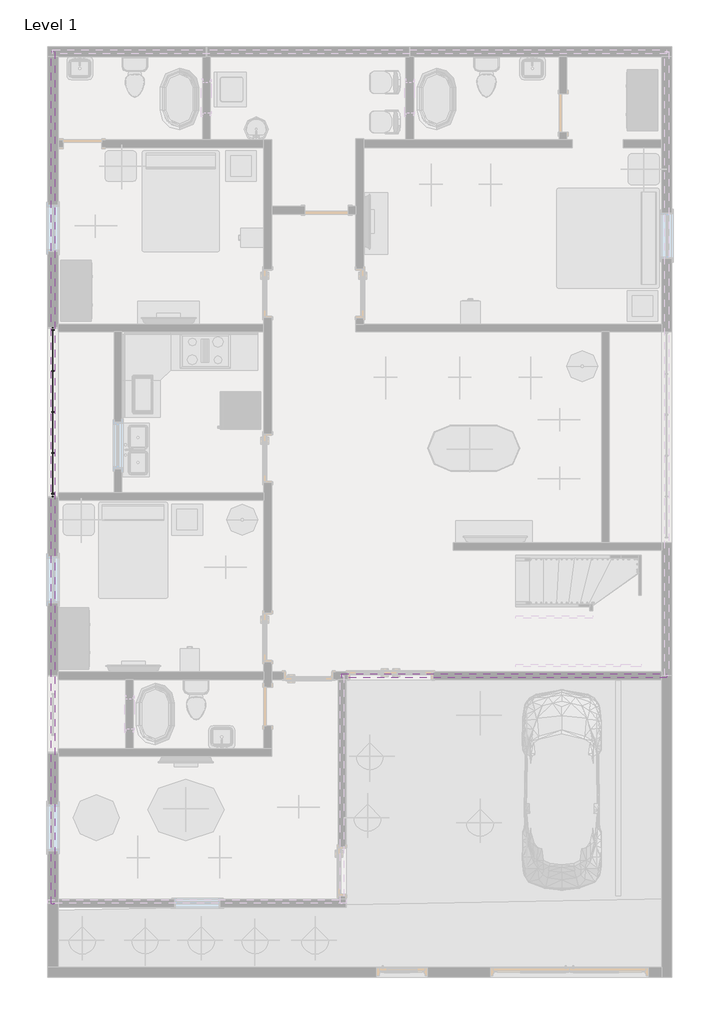
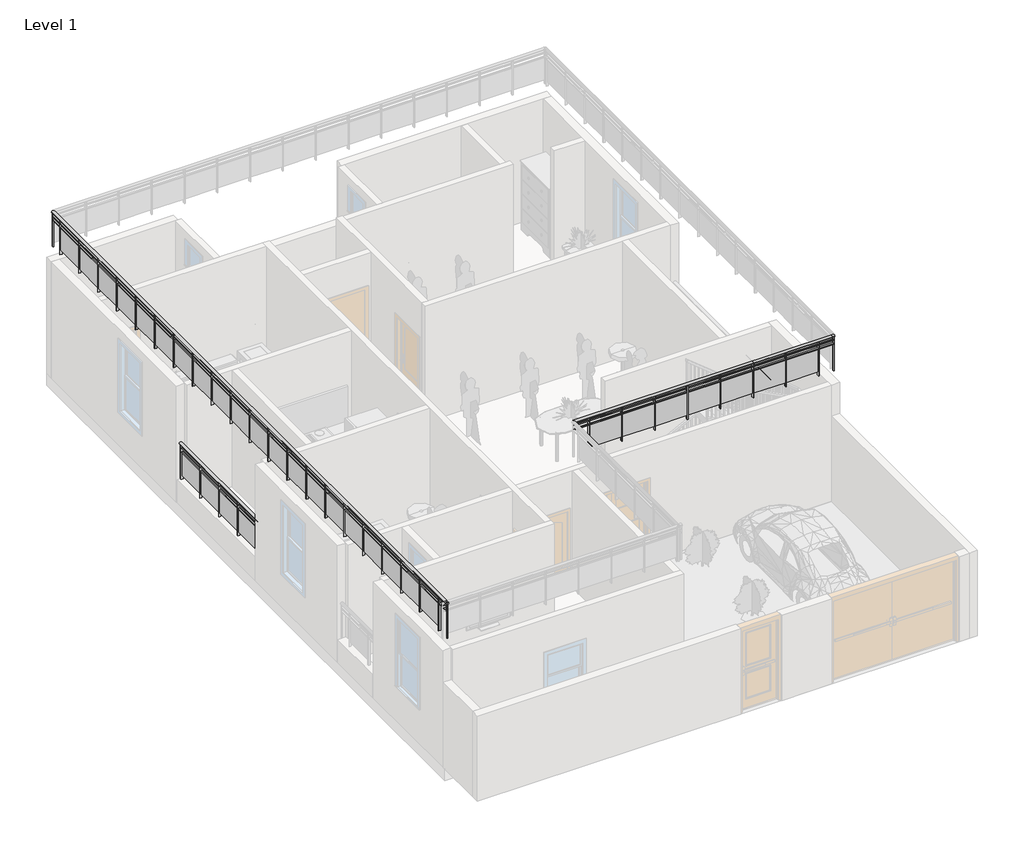
# One storey, part 3 of 6: 3 railings.
"""IFC4 building model written with IfcOpenShell, lengths in millimetres."""

from ifc_helpers import new_model, si_unit, point, frame, origin, place, context, project, spatial, polyline, ellipse_curve, trimmed, outline, extrude, element, save
from ifc_brep_helpers import plane_surface, extruded_surface, advanced_brep

model = new_model("IFC4")

# Units and contexts
model_context = context("Model", 3, world=origin())
ifc_project = project(units=[si_unit("LENGTHUNIT", "METRE", prefix="MILLI")], contexts=[model_context])

# Site, building, storey
site = spatial("IfcSite", under=ifc_project)
building = spatial("IfcBuilding", under=site)
storey = spatial("IfcBuildingStorey", under=building, Name="Level 1", Elevation=0.0)

# Railings
placement = place(None, origin())
element("IfcRailing", 1, ObjectType="Glass Panel - Bottom Fill", at=placement, inside=storey, context=model_context, shape_type="SolidModel", body=[
    advanced_brep(
    [(-14543.6841185, 4912.4271763, 1524.0), (-14467.4841185, 4912.4271763, 1524.0), (-14543.6841185, 8277.9271763, 1524.0), (-14467.4841185, 8277.9271763, 1524.0)],
    [
        (0, 1, ellipse_curve(frame((-14505.5841185, 4912.4271763, 1524.0), z_axis=(0.0, -1.0, 0.0), x_axis=(1.0, 0.0, 0.0)), 38.1, 28.575)),
        (1, 0, ellipse_curve(frame((-14505.5841185, 4912.4271763, 1524.0), z_axis=(0.0, -1.0, 0.0), x_axis=(1.0, 0.0, 0.0)), 38.1, 28.575)),
        (2, 3, ellipse_curve(frame((-14505.5841185, 8277.9271763, 1524.0), z_axis=(0.0, 1.0, 0.0), x_axis=(1.0, 0.0, 0.0)), 38.1, 28.575)),
        (3, 2, ellipse_curve(frame((-14505.5841185, 8277.9271763, 1524.0), z_axis=(0.0, 1.0, 0.0), x_axis=(1.0, 0.0, 0.0)), 38.1, 28.575)),
        (0, 2),
        (3, 1),
    ],
    [
        plane_surface(frame((-14505.5841185, 4912.4271763, 1524.0), z_axis=(0.0, -1.0, 0.0), x_axis=(0.0, 0.0, 1.0))),
        plane_surface(frame((-14505.5841185, 8277.9271763, 1524.0), z_axis=(0.0, 1.0, 0.0), x_axis=(0.0, 0.0, 1.0))),
        extruded_surface(trimmed(ellipse_curve(frame((-14505.5841185, 8277.9271763, 1524.0), z_axis=(0.0, -1.0, 0.0), x_axis=(1.0, 0.0, 0.0)), 38.1, 28.575), [point((-14543.6841185, 8277.9271763, 1524.0))], [point((-14467.4841185, 8277.9271763, 1524.0))], True, "CARTESIAN"), (0.0, -3365.5, 0.0), 3365.5),
        extruded_surface(trimmed(ellipse_curve(frame((-14505.5841185, 8277.9271763, 1524.0), z_axis=(0.0, -1.0, 0.0), x_axis=(1.0, 0.0, 0.0)), 38.1, 28.575), [point((-14467.4841185, 8277.9271763, 1524.0))], [point((-14543.6841185, 8277.9271763, 1524.0))], True, "CARTESIAN"), (0.0, -3365.5, 0.0), 3365.5),
    ],
    [
        (0, [[1, 2]]),
        (1, [[3, 4]]),
        (2, [[-1, 5, -4, 6]]),
        (3, [[-2, -6, -3, -5]]),
    ],
),
    extrude(outline(polyline([(-14492.8841185, 4912.4271763), (-14518.2841185, 4912.4271763), (-14518.2841185, 8277.9271763), (-14492.8841185, 8277.9271763), (-14492.8841185, 4912.4271763)])), frame((0.0, 0.0, 1409.7), z_axis=(0.0, 0.0, 1.0), x_axis=(1.0, 0.0, 0.0)), (0.0, 0.0, 1.0), 25.4),
    extrude(outline(polyline([(-14492.8841185, 4912.4271763), (-14518.2841185, 4912.4271763), (-14518.2841185, 8277.9271763), (-14492.8841185, 8277.9271763), (-14492.8841185, 4912.4271763)])), frame((0.0, 0.0, 1308.1), z_axis=(0.0, 0.0, 1.0), x_axis=(1.0, 0.0, 0.0)), (0.0, 0.0, 1.0), 25.4),
    extrude(outline(polyline([(-14480.1841185, 8214.4271763), (-14530.9841185, 8214.4271763), (-14530.9841185, 8227.1271763), (-14480.1841185, 8227.1271763), (-14480.1841185, 8214.4271763)])), frame((0.0, 0.0, 609.6), z_axis=(0.0, 0.0, 1.0), x_axis=(1.0, 0.0, 0.0)), (0.0, 0.0, 1.0), 885.6788223),
    extrude(outline(polyline([(-14512.1192755, 7407.9771763), (-14512.1192755, 8220.7771763), (-14505.7692755, 8220.7771763), (-14505.7692755, 7407.9771763), (-14512.1192755, 7407.9771763)])), frame((0.0, 0.0, 711.2), z_axis=(0.0, 0.0, 1.0), x_axis=(1.0, 0.0, 0.0)), (0.0, 0.0, 1.0), 596.9),
    extrude(outline(polyline([(-14480.1841185, 7401.6271763), (-14530.9841185, 7401.6271763), (-14530.9841185, 7414.3271763), (-14480.1841185, 7414.3271763), (-14480.1841185, 7401.6271763)])), frame((0.0, 0.0, 609.6), z_axis=(0.0, 0.0, 1.0), x_axis=(1.0, 0.0, 0.0)), (0.0, 0.0, 1.0), 885.6788223),
    extrude(outline(polyline([(-14512.1192755, 6595.1771763), (-14512.1192755, 7407.9771763), (-14505.7692755, 7407.9771763), (-14505.7692755, 6595.1771763), (-14512.1192755, 6595.1771763)])), frame((0.0, 0.0, 711.2), z_axis=(0.0, 0.0, 1.0), x_axis=(1.0, 0.0, 0.0)), (0.0, 0.0, 1.0), 596.9),
    extrude(outline(polyline([(-14480.1841185, 6588.8271763), (-14530.9841185, 6588.8271763), (-14530.9841185, 6601.5271763), (-14480.1841185, 6601.5271763), (-14480.1841185, 6588.8271763)])), frame((0.0, 0.0, 609.6), z_axis=(0.0, 0.0, 1.0), x_axis=(1.0, 0.0, 0.0)), (0.0, 0.0, 1.0), 885.6788223),
    extrude(outline(polyline([(-14512.1192755, 5782.3771763), (-14512.1192755, 6595.1771763), (-14505.7692755, 6595.1771763), (-14505.7692755, 5782.3771763), (-14512.1192755, 5782.3771763)])), frame((0.0, 0.0, 711.2), z_axis=(0.0, 0.0, 1.0), x_axis=(1.0, 0.0, 0.0)), (0.0, 0.0, 1.0), 596.9),
    extrude(outline(polyline([(-14480.1841185, 5776.0271763), (-14530.9841185, 5776.0271763), (-14530.9841185, 5788.7271763), (-14480.1841185, 5788.7271763), (-14480.1841185, 5776.0271763)])), frame((0.0, 0.0, 609.6), z_axis=(0.0, 0.0, 1.0), x_axis=(1.0, 0.0, 0.0)), (0.0, 0.0, 1.0), 885.6788223),
    extrude(outline(polyline([(-14512.1192755, 4969.5771763), (-14512.1192755, 5782.3771763), (-14505.7692755, 5782.3771763), (-14505.7692755, 4969.5771763), (-14512.1192755, 4969.5771763)])), frame((0.0, 0.0, 711.2), z_axis=(0.0, 0.0, 1.0), x_axis=(1.0, 0.0, 0.0)), (0.0, 0.0, 1.0), 596.9),
    extrude(outline(polyline([(-14480.1841185, 4963.2271763), (-14530.9841185, 4963.2271763), (-14530.9841185, 4975.9271763), (-14480.1841185, 4975.9271763), (-14480.1841185, 4963.2271763)])), frame((0.0, 0.0, 609.6), z_axis=(0.0, 0.0, 1.0), x_axis=(1.0, 0.0, 0.0)), (0.0, 0.0, 1.0), 885.6788223),
    extrude(outline(polyline([(-14496.0591185, 8265.2271763), (-14515.1091185, 8265.2271763), (-14515.1091185, 8284.2771763), (-14496.0591185, 8284.2771763), (-14496.0591185, 8265.2271763)])), frame((0.0, 0.0, 609.6), z_axis=(0.0, 0.0, 1.0), x_axis=(1.0, 0.0, 0.0)), (0.0, 0.0, 1.0), 885.6788223),
    extrude(outline(polyline([(-14496.0591185, 4906.0771763), (-14515.1091185, 4906.0771763), (-14515.1091185, 4925.1271763), (-14496.0591185, 4925.1271763), (-14496.0591185, 4906.0771763)])), frame((0.0, 0.0, 609.6), z_axis=(0.0, 0.0, 1.0), x_axis=(1.0, 0.0, 0.0)), (0.0, 0.0, 1.0), 885.6788223),
])
element("IfcRailing", 2, ObjectType="Glass Panel - Bottom Fill", at=placement, inside=storey, context=model_context, shape_type="SolidModel", body=[
    advanced_brep(
    [(-2313.5841185, 1318.3271763, 4267.2), (-2313.5841185, 1394.5271763, 4267.2), (-8765.1841185, 1318.3271763, 4267.2), (-8765.1841185, 1394.5271763, 4267.2)],
    [
        (0, 1, ellipse_curve(frame((-2313.5841185, 1356.4271763, 4267.2), z_axis=(1.0, 0.0, 0.0), x_axis=(0.0, 1.0, 0.0)), 38.1, 28.575)),
        (1, 0, ellipse_curve(frame((-2313.5841185, 1356.4271763, 4267.2), z_axis=(1.0, 0.0, 0.0), x_axis=(0.0, 1.0, 0.0)), 38.1, 28.575)),
        (2, 3, ellipse_curve(frame((-8765.1841185, 1356.4271763, 4267.2), z_axis=(-1.0, 0.0, 0.0), x_axis=(0.0, 1.0, 0.0)), 38.1, 28.575)),
        (3, 2, ellipse_curve(frame((-8765.1841185, 1356.4271763, 4267.2), z_axis=(-1.0, 0.0, 0.0), x_axis=(0.0, 1.0, 0.0)), 38.1, 28.575)),
        (0, 2),
        (3, 1),
    ],
    [
        plane_surface(frame((-2313.5841185, 1356.4271763, 4267.2), z_axis=(1.0, 0.0, 0.0), x_axis=(0.0, -1.0, 0.0))),
        plane_surface(frame((-8765.1841185, 1356.4271763, 4267.2), z_axis=(-1.0, 0.0, 0.0), x_axis=(0.0, -1.0, 0.0))),
        extruded_surface(trimmed(ellipse_curve(frame((-8765.1841185, 1356.4271763, 4267.2), z_axis=(1.0, 0.0, 0.0), x_axis=(0.0, 1.0, 0.0)), 38.1, 28.575), [point((-8765.1841185, 1318.3271763, 4267.2))], [point((-8765.1841185, 1394.5271763, 4267.2))], True, "CARTESIAN"), (6451.599999999999, 0.0, 0.0), 6451.599999999999),
        extruded_surface(trimmed(ellipse_curve(frame((-8765.1841185, 1356.4271763, 4267.2), z_axis=(1.0, 0.0, 0.0), x_axis=(0.0, 1.0, 0.0)), 38.1, 28.575), [point((-8765.1841185, 1394.5271763, 4267.2))], [point((-8765.1841185, 1318.3271763, 4267.2))], True, "CARTESIAN"), (6451.599999999999, 0.0, 0.0), 6451.599999999999),
    ],
    [
        (0, [[1, 2]]),
        (1, [[3, 4]]),
        (2, [[-1, 5, -4, 6]]),
        (3, [[-2, -6, -3, -5]]),
    ],
),
    extrude(outline(polyline([(-2313.5841185, 1369.1271763), (-2313.5841185, 1343.7271763), (-8765.1841185, 1343.7271763), (-8765.1841185, 1369.1271763), (-2313.5841185, 1369.1271763)])), frame((0.0, 0.0, 4152.9), z_axis=(0.0, 0.0, 1.0), x_axis=(1.0, 0.0, 0.0)), (0.0, 0.0, 1.0), 25.4),
    extrude(outline(polyline([(-2313.5841185, 1369.1271763), (-2313.5841185, 1343.7271763), (-8765.1841185, 1343.7271763), (-8765.1841185, 1369.1271763), (-2313.5841185, 1369.1271763)])), frame((0.0, 0.0, 4051.3), z_axis=(0.0, 0.0, 1.0), x_axis=(1.0, 0.0, 0.0)), (0.0, 0.0, 1.0), 25.4),
    extrude(outline(polyline([(-8377.8341185, 1381.8271763), (-8377.8341185, 1331.0271763), (-8390.5341185, 1331.0271763), (-8390.5341185, 1381.8271763), (-8377.8341185, 1381.8271763)])), frame((0.0, 0.0, 3352.8), z_axis=(0.0, 0.0, 1.0), x_axis=(1.0, 0.0, 0.0)), (0.0, 0.0, 1.0), 885.6788223),
    extrude(outline(polyline([(-7571.3841185, 1349.8920193), (-8384.1841185, 1349.8920193), (-8384.1841185, 1356.2420193), (-7571.3841185, 1356.2420193), (-7571.3841185, 1349.8920193)])), frame((0.0, 0.0, 3454.4), z_axis=(0.0, 0.0, 1.0), x_axis=(1.0, 0.0, 0.0)), (0.0, 0.0, 1.0), 596.9),
    extrude(outline(polyline([(-7565.0341185, 1381.8271763), (-7565.0341185, 1331.0271763), (-7577.7341185, 1331.0271763), (-7577.7341185, 1381.8271763), (-7565.0341185, 1381.8271763)])), frame((0.0, 0.0, 3352.8), z_axis=(0.0, 0.0, 1.0), x_axis=(1.0, 0.0, 0.0)), (0.0, 0.0, 1.0), 885.6788223),
    extrude(outline(polyline([(-6758.5841185, 1349.8920193), (-7571.3841185, 1349.8920193), (-7571.3841185, 1356.2420193), (-6758.5841185, 1356.2420193), (-6758.5841185, 1349.8920193)])), frame((0.0, 0.0, 3454.4), z_axis=(0.0, 0.0, 1.0), x_axis=(1.0, 0.0, 0.0)), (0.0, 0.0, 1.0), 596.9),
    extrude(outline(polyline([(-6752.2341185, 1381.8271763), (-6752.2341185, 1331.0271763), (-6764.9341185, 1331.0271763), (-6764.9341185, 1381.8271763), (-6752.2341185, 1381.8271763)])), frame((0.0, 0.0, 3352.8), z_axis=(0.0, 0.0, 1.0), x_axis=(1.0, 0.0, 0.0)), (0.0, 0.0, 1.0), 885.6788223),
    extrude(outline(polyline([(-5945.7841185, 1349.8920193), (-6758.5841185, 1349.8920193), (-6758.5841185, 1356.2420193), (-5945.7841185, 1356.2420193), (-5945.7841185, 1349.8920193)])), frame((0.0, 0.0, 3454.4), z_axis=(0.0, 0.0, 1.0), x_axis=(1.0, 0.0, 0.0)), (0.0, 0.0, 1.0), 596.9),
    extrude(outline(polyline([(-5939.4341185, 1381.8271763), (-5939.4341185, 1331.0271763), (-5952.1341185, 1331.0271763), (-5952.1341185, 1381.8271763), (-5939.4341185, 1381.8271763)])), frame((0.0, 0.0, 3352.8), z_axis=(0.0, 0.0, 1.0), x_axis=(1.0, 0.0, 0.0)), (0.0, 0.0, 1.0), 885.6788223),
    extrude(outline(polyline([(-5132.9841185, 1349.8920193), (-5945.7841185, 1349.8920193), (-5945.7841185, 1356.2420193), (-5132.9841185, 1356.2420193), (-5132.9841185, 1349.8920193)])), frame((0.0, 0.0, 3454.4), z_axis=(0.0, 0.0, 1.0), x_axis=(1.0, 0.0, 0.0)), (0.0, 0.0, 1.0), 596.9),
    extrude(outline(polyline([(-5126.6341185, 1381.8271763), (-5126.6341185, 1331.0271763), (-5139.3341185, 1331.0271763), (-5139.3341185, 1381.8271763), (-5126.6341185, 1381.8271763)])), frame((0.0, 0.0, 3352.8), z_axis=(0.0, 0.0, 1.0), x_axis=(1.0, 0.0, 0.0)), (0.0, 0.0, 1.0), 885.6788223),
    extrude(outline(polyline([(-4320.1841185, 1349.8920193), (-5132.9841185, 1349.8920193), (-5132.9841185, 1356.2420193), (-4320.1841185, 1356.2420193), (-4320.1841185, 1349.8920193)])), frame((0.0, 0.0, 3454.4), z_axis=(0.0, 0.0, 1.0), x_axis=(1.0, 0.0, 0.0)), (0.0, 0.0, 1.0), 596.9),
    extrude(outline(polyline([(-4313.8341185, 1381.8271763), (-4313.8341185, 1331.0271763), (-4326.5341185, 1331.0271763), (-4326.5341185, 1381.8271763), (-4313.8341185, 1381.8271763)])), frame((0.0, 0.0, 3352.8), z_axis=(0.0, 0.0, 1.0), x_axis=(1.0, 0.0, 0.0)), (0.0, 0.0, 1.0), 885.6788223),
    extrude(outline(polyline([(-3507.3841185, 1349.8920193), (-4320.1841185, 1349.8920193), (-4320.1841185, 1356.2420193), (-3507.3841185, 1356.2420193), (-3507.3841185, 1349.8920193)])), frame((0.0, 0.0, 3454.4), z_axis=(0.0, 0.0, 1.0), x_axis=(1.0, 0.0, 0.0)), (0.0, 0.0, 1.0), 596.9),
    extrude(outline(polyline([(-3501.0341185, 1381.8271763), (-3501.0341185, 1331.0271763), (-3513.7341185, 1331.0271763), (-3513.7341185, 1381.8271763), (-3501.0341185, 1381.8271763)])), frame((0.0, 0.0, 3352.8), z_axis=(0.0, 0.0, 1.0), x_axis=(1.0, 0.0, 0.0)), (0.0, 0.0, 1.0), 885.6788223),
    extrude(outline(polyline([(-2694.5841185, 1349.8920193), (-3507.3841185, 1349.8920193), (-3507.3841185, 1356.2420193), (-2694.5841185, 1356.2420193), (-2694.5841185, 1349.8920193)])), frame((0.0, 0.0, 3454.4), z_axis=(0.0, 0.0, 1.0), x_axis=(1.0, 0.0, 0.0)), (0.0, 0.0, 1.0), 596.9),
    extrude(outline(polyline([(-2688.2341185, 1381.8271763), (-2688.2341185, 1331.0271763), (-2700.9341185, 1331.0271763), (-2700.9341185, 1381.8271763), (-2688.2341185, 1381.8271763)])), frame((0.0, 0.0, 3352.8), z_axis=(0.0, 0.0, 1.0), x_axis=(1.0, 0.0, 0.0)), (0.0, 0.0, 1.0), 885.6788223),
    extrude(outline(polyline([(-8752.4841185, 1365.9521763), (-8752.4841185, 1346.9021763), (-8771.5341185, 1346.9021763), (-8771.5341185, 1365.9521763), (-8752.4841185, 1365.9521763)])), frame((0.0, 0.0, 3352.8), z_axis=(0.0, 0.0, 1.0), x_axis=(1.0, 0.0, 0.0)), (0.0, 0.0, 1.0), 885.6788223),
    extrude(outline(polyline([(-2307.2341185, 1365.9521763), (-2307.2341185, 1346.9021763), (-2326.2841185, 1346.9021763), (-2326.2841185, 1365.9521763), (-2307.2341185, 1365.9521763)])), frame((0.0, 0.0, 3352.8), z_axis=(0.0, 0.0, 1.0), x_axis=(1.0, 0.0, 0.0)), (0.0, 0.0, 1.0), 885.6788223),
])
element("IfcRailing", 3, ObjectType="Glass Panel - Bottom Fill", at=placement, inside=storey, context=model_context, shape_type="SolidModel", body=[
    advanced_brep(
    [(-14543.6841185, -3177.4728237, 4267.2), (-14467.4841185, -3177.4728237, 4267.2), (-14543.6841185, 13751.6271763, 4267.2), (-14467.4841185, 13751.6271763, 4267.2)],
    [
        (0, 1, ellipse_curve(frame((-14505.5841185, -3177.4728237, 4267.2), z_axis=(0.0, -1.0, 0.0), x_axis=(1.0, 0.0, 0.0)), 38.1, 28.575)),
        (1, 0, ellipse_curve(frame((-14505.5841185, -3177.4728237, 4267.2), z_axis=(0.0, -1.0, 0.0), x_axis=(1.0, 0.0, 0.0)), 38.1, 28.575)),
        (2, 3, ellipse_curve(frame((-14505.5841185, 13751.6271763, 4267.2), z_axis=(0.0, 1.0, 0.0), x_axis=(1.0, 0.0, 0.0)), 38.1, 28.575)),
        (3, 2, ellipse_curve(frame((-14505.5841185, 13751.6271763, 4267.2), z_axis=(0.0, 1.0, 0.0), x_axis=(1.0, 0.0, 0.0)), 38.1, 28.575)),
        (0, 2),
        (3, 1),
    ],
    [
        plane_surface(frame((-14505.5841185, -3177.4728237, 4267.2), z_axis=(0.0, -1.0, 0.0), x_axis=(0.0, 0.0, 1.0))),
        plane_surface(frame((-14505.5841185, 13751.6271763, 4267.2), z_axis=(0.0, 1.0, 0.0), x_axis=(0.0, 0.0, 1.0))),
        extruded_surface(trimmed(ellipse_curve(frame((-14505.5841185, 13751.6271763, 4267.2), z_axis=(0.0, -1.0, 0.0), x_axis=(1.0, 0.0, 0.0)), 38.1, 28.575), [point((-14543.6841185, 13751.6271763, 4267.2))], [point((-14467.4841185, 13751.6271763, 4267.2))], True, "CARTESIAN"), (0.0, -16929.1, 0.0), 16929.1),
        extruded_surface(trimmed(ellipse_curve(frame((-14505.5841185, 13751.6271763, 4267.2), z_axis=(0.0, -1.0, 0.0), x_axis=(1.0, 0.0, 0.0)), 38.1, 28.575), [point((-14467.4841185, 13751.6271763, 4267.2))], [point((-14543.6841185, 13751.6271763, 4267.2))], True, "CARTESIAN"), (0.0, -16929.1, 0.0), 16929.1),
    ],
    [
        (0, [[1, 2]]),
        (1, [[3, 4]]),
        (2, [[-1, 5, -4, 6]]),
        (3, [[-2, -6, -3, -5]]),
    ],
),
    extrude(outline(polyline([(-14492.8841185, -3177.4728237), (-14518.2841185, -3177.4728237), (-14518.2841185, 13751.6271763), (-14492.8841185, 13751.6271763), (-14492.8841185, -3177.4728237)])), frame((0.0, 0.0, 4152.9), z_axis=(0.0, 0.0, 1.0), x_axis=(1.0, 0.0, 0.0)), (0.0, 0.0, 1.0), 25.4),
    extrude(outline(polyline([(-14492.8841185, -3177.4728237), (-14518.2841185, -3177.4728237), (-14518.2841185, 13751.6271763), (-14492.8841185, 13751.6271763), (-14492.8841185, -3177.4728237)])), frame((0.0, 0.0, 4051.3), z_axis=(0.0, 0.0, 1.0), x_axis=(1.0, 0.0, 0.0)), (0.0, 0.0, 1.0), 25.4),
    extrude(outline(polyline([(-14480.1841185, 13408.7271763), (-14530.9841185, 13408.7271763), (-14530.9841185, 13421.4271763), (-14480.1841185, 13421.4271763), (-14480.1841185, 13408.7271763)])), frame((0.0, 0.0, 3352.8), z_axis=(0.0, 0.0, 1.0), x_axis=(1.0, 0.0, 0.0)), (0.0, 0.0, 1.0), 885.6788223),
    extrude(outline(polyline([(-14512.1192755, 12602.2771763), (-14512.1192755, 13415.0771763), (-14505.7692755, 13415.0771763), (-14505.7692755, 12602.2771763), (-14512.1192755, 12602.2771763)])), frame((0.0, 0.0, 3454.4), z_axis=(0.0, 0.0, 1.0), x_axis=(1.0, 0.0, 0.0)), (0.0, 0.0, 1.0), 596.9),
    extrude(outline(polyline([(-14480.1841185, 12595.9271763), (-14530.9841185, 12595.9271763), (-14530.9841185, 12608.6271763), (-14480.1841185, 12608.6271763), (-14480.1841185, 12595.9271763)])), frame((0.0, 0.0, 3352.8), z_axis=(0.0, 0.0, 1.0), x_axis=(1.0, 0.0, 0.0)), (0.0, 0.0, 1.0), 885.6788223),
    extrude(outline(polyline([(-14512.1192755, 11789.4771763), (-14512.1192755, 12602.2771763), (-14505.7692755, 12602.2771763), (-14505.7692755, 11789.4771763), (-14512.1192755, 11789.4771763)])), frame((0.0, 0.0, 3454.4), z_axis=(0.0, 0.0, 1.0), x_axis=(1.0, 0.0, 0.0)), (0.0, 0.0, 1.0), 596.9),
    extrude(outline(polyline([(-14480.1841185, 11783.1271763), (-14530.9841185, 11783.1271763), (-14530.9841185, 11795.8271763), (-14480.1841185, 11795.8271763), (-14480.1841185, 11783.1271763)])), frame((0.0, 0.0, 3352.8), z_axis=(0.0, 0.0, 1.0), x_axis=(1.0, 0.0, 0.0)), (0.0, 0.0, 1.0), 885.6788223),
    extrude(outline(polyline([(-14512.1192755, 10976.6771763), (-14512.1192755, 11789.4771763), (-14505.7692755, 11789.4771763), (-14505.7692755, 10976.6771763), (-14512.1192755, 10976.6771763)])), frame((0.0, 0.0, 3454.4), z_axis=(0.0, 0.0, 1.0), x_axis=(1.0, 0.0, 0.0)), (0.0, 0.0, 1.0), 596.9),
    extrude(outline(polyline([(-14480.1841185, 10970.3271763), (-14530.9841185, 10970.3271763), (-14530.9841185, 10983.0271763), (-14480.1841185, 10983.0271763), (-14480.1841185, 10970.3271763)])), frame((0.0, 0.0, 3352.8), z_axis=(0.0, 0.0, 1.0), x_axis=(1.0, 0.0, 0.0)), (0.0, 0.0, 1.0), 885.6788223),
    extrude(outline(polyline([(-14512.1192755, 10163.8771763), (-14512.1192755, 10976.6771763), (-14505.7692755, 10976.6771763), (-14505.7692755, 10163.8771763), (-14512.1192755, 10163.8771763)])), frame((0.0, 0.0, 3454.4), z_axis=(0.0, 0.0, 1.0), x_axis=(1.0, 0.0, 0.0)), (0.0, 0.0, 1.0), 596.9),
    extrude(outline(polyline([(-14480.1841185, 10157.5271763), (-14530.9841185, 10157.5271763), (-14530.9841185, 10170.2271763), (-14480.1841185, 10170.2271763), (-14480.1841185, 10157.5271763)])), frame((0.0, 0.0, 3352.8), z_axis=(0.0, 0.0, 1.0), x_axis=(1.0, 0.0, 0.0)), (0.0, 0.0, 1.0), 885.6788223),
    extrude(outline(polyline([(-14512.1192755, 9351.0771763), (-14512.1192755, 10163.8771763), (-14505.7692755, 10163.8771763), (-14505.7692755, 9351.0771763), (-14512.1192755, 9351.0771763)])), frame((0.0, 0.0, 3454.4), z_axis=(0.0, 0.0, 1.0), x_axis=(1.0, 0.0, 0.0)), (0.0, 0.0, 1.0), 596.9),
    extrude(outline(polyline([(-14480.1841185, 9344.7271763), (-14530.9841185, 9344.7271763), (-14530.9841185, 9357.4271763), (-14480.1841185, 9357.4271763), (-14480.1841185, 9344.7271763)])), frame((0.0, 0.0, 3352.8), z_axis=(0.0, 0.0, 1.0), x_axis=(1.0, 0.0, 0.0)), (0.0, 0.0, 1.0), 885.6788223),
    extrude(outline(polyline([(-14512.1192755, 8538.2771763), (-14512.1192755, 9351.0771763), (-14505.7692755, 9351.0771763), (-14505.7692755, 8538.2771763), (-14512.1192755, 8538.2771763)])), frame((0.0, 0.0, 3454.4), z_axis=(0.0, 0.0, 1.0), x_axis=(1.0, 0.0, 0.0)), (0.0, 0.0, 1.0), 596.9),
    extrude(outline(polyline([(-14480.1841185, 8531.9271763), (-14530.9841185, 8531.9271763), (-14530.9841185, 8544.6271763), (-14480.1841185, 8544.6271763), (-14480.1841185, 8531.9271763)])), frame((0.0, 0.0, 3352.8), z_axis=(0.0, 0.0, 1.0), x_axis=(1.0, 0.0, 0.0)), (0.0, 0.0, 1.0), 885.6788223),
    extrude(outline(polyline([(-14512.1192755, 7725.4771763), (-14512.1192755, 8538.2771763), (-14505.7692755, 8538.2771763), (-14505.7692755, 7725.4771763), (-14512.1192755, 7725.4771763)])), frame((0.0, 0.0, 3454.4), z_axis=(0.0, 0.0, 1.0), x_axis=(1.0, 0.0, 0.0)), (0.0, 0.0, 1.0), 596.9),
    extrude(outline(polyline([(-14480.1841185, 7719.1271763), (-14530.9841185, 7719.1271763), (-14530.9841185, 7731.8271763), (-14480.1841185, 7731.8271763), (-14480.1841185, 7719.1271763)])), frame((0.0, 0.0, 3352.8), z_axis=(0.0, 0.0, 1.0), x_axis=(1.0, 0.0, 0.0)), (0.0, 0.0, 1.0), 885.6788223),
    extrude(outline(polyline([(-14512.1192755, 6912.6771763), (-14512.1192755, 7725.4771763), (-14505.7692755, 7725.4771763), (-14505.7692755, 6912.6771763), (-14512.1192755, 6912.6771763)])), frame((0.0, 0.0, 3454.4), z_axis=(0.0, 0.0, 1.0), x_axis=(1.0, 0.0, 0.0)), (0.0, 0.0, 1.0), 596.9),
    extrude(outline(polyline([(-14480.1841185, 6906.3271763), (-14530.9841185, 6906.3271763), (-14530.9841185, 6919.0271763), (-14480.1841185, 6919.0271763), (-14480.1841185, 6906.3271763)])), frame((0.0, 0.0, 3352.8), z_axis=(0.0, 0.0, 1.0), x_axis=(1.0, 0.0, 0.0)), (0.0, 0.0, 1.0), 885.6788223),
    extrude(outline(polyline([(-14512.1192755, 6099.8771763), (-14512.1192755, 6912.6771763), (-14505.7692755, 6912.6771763), (-14505.7692755, 6099.8771763), (-14512.1192755, 6099.8771763)])), frame((0.0, 0.0, 3454.4), z_axis=(0.0, 0.0, 1.0), x_axis=(1.0, 0.0, 0.0)), (0.0, 0.0, 1.0), 596.9),
    extrude(outline(polyline([(-14480.1841185, 6093.5271763), (-14530.9841185, 6093.5271763), (-14530.9841185, 6106.2271763), (-14480.1841185, 6106.2271763), (-14480.1841185, 6093.5271763)])), frame((0.0, 0.0, 3352.8), z_axis=(0.0, 0.0, 1.0), x_axis=(1.0, 0.0, 0.0)), (0.0, 0.0, 1.0), 885.6788223),
    extrude(outline(polyline([(-14512.1192755, 5287.0771763), (-14512.1192755, 6099.8771763), (-14505.7692755, 6099.8771763), (-14505.7692755, 5287.0771763), (-14512.1192755, 5287.0771763)])), frame((0.0, 0.0, 3454.4), z_axis=(0.0, 0.0, 1.0), x_axis=(1.0, 0.0, 0.0)), (0.0, 0.0, 1.0), 596.9),
    extrude(outline(polyline([(-14480.1841185, 5280.7271763), (-14530.9841185, 5280.7271763), (-14530.9841185, 5293.4271763), (-14480.1841185, 5293.4271763), (-14480.1841185, 5280.7271763)])), frame((0.0, 0.0, 3352.8), z_axis=(0.0, 0.0, 1.0), x_axis=(1.0, 0.0, 0.0)), (0.0, 0.0, 1.0), 885.6788223),
    extrude(outline(polyline([(-14512.1192755, 4474.2771763), (-14512.1192755, 5287.0771763), (-14505.7692755, 5287.0771763), (-14505.7692755, 4474.2771763), (-14512.1192755, 4474.2771763)])), frame((0.0, 0.0, 3454.4), z_axis=(0.0, 0.0, 1.0), x_axis=(1.0, 0.0, 0.0)), (0.0, 0.0, 1.0), 596.9),
    extrude(outline(polyline([(-14480.1841185, 4467.9271763), (-14530.9841185, 4467.9271763), (-14530.9841185, 4480.6271763), (-14480.1841185, 4480.6271763), (-14480.1841185, 4467.9271763)])), frame((0.0, 0.0, 3352.8), z_axis=(0.0, 0.0, 1.0), x_axis=(1.0, 0.0, 0.0)), (0.0, 0.0, 1.0), 885.6788223),
    extrude(outline(polyline([(-14512.1192755, 3661.4771763), (-14512.1192755, 4474.2771763), (-14505.7692755, 4474.2771763), (-14505.7692755, 3661.4771763), (-14512.1192755, 3661.4771763)])), frame((0.0, 0.0, 3454.4), z_axis=(0.0, 0.0, 1.0), x_axis=(1.0, 0.0, 0.0)), (0.0, 0.0, 1.0), 596.9),
    extrude(outline(polyline([(-14480.1841185, 3655.1271763), (-14530.9841185, 3655.1271763), (-14530.9841185, 3667.8271763), (-14480.1841185, 3667.8271763), (-14480.1841185, 3655.1271763)])), frame((0.0, 0.0, 3352.8), z_axis=(0.0, 0.0, 1.0), x_axis=(1.0, 0.0, 0.0)), (0.0, 0.0, 1.0), 885.6788223),
    extrude(outline(polyline([(-14512.1192755, 2848.6771763), (-14512.1192755, 3661.4771763), (-14505.7692755, 3661.4771763), (-14505.7692755, 2848.6771763), (-14512.1192755, 2848.6771763)])), frame((0.0, 0.0, 3454.4), z_axis=(0.0, 0.0, 1.0), x_axis=(1.0, 0.0, 0.0)), (0.0, 0.0, 1.0), 596.9),
    extrude(outline(polyline([(-14480.1841185, 2842.3271763), (-14530.9841185, 2842.3271763), (-14530.9841185, 2855.0271763), (-14480.1841185, 2855.0271763), (-14480.1841185, 2842.3271763)])), frame((0.0, 0.0, 3352.8), z_axis=(0.0, 0.0, 1.0), x_axis=(1.0, 0.0, 0.0)), (0.0, 0.0, 1.0), 885.6788223),
    extrude(outline(polyline([(-14512.1192755, 2035.8771763), (-14512.1192755, 2848.6771763), (-14505.7692755, 2848.6771763), (-14505.7692755, 2035.8771763), (-14512.1192755, 2035.8771763)])), frame((0.0, 0.0, 3454.4), z_axis=(0.0, 0.0, 1.0), x_axis=(1.0, 0.0, 0.0)), (0.0, 0.0, 1.0), 596.9),
    extrude(outline(polyline([(-14480.1841185, 2029.5271763), (-14530.9841185, 2029.5271763), (-14530.9841185, 2042.2271763), (-14480.1841185, 2042.2271763), (-14480.1841185, 2029.5271763)])), frame((0.0, 0.0, 3352.8), z_axis=(0.0, 0.0, 1.0), x_axis=(1.0, 0.0, 0.0)), (0.0, 0.0, 1.0), 885.6788223),
    extrude(outline(polyline([(-14512.1192755, 1223.0771763), (-14512.1192755, 2035.8771763), (-14505.7692755, 2035.8771763), (-14505.7692755, 1223.0771763), (-14512.1192755, 1223.0771763)])), frame((0.0, 0.0, 3454.4), z_axis=(0.0, 0.0, 1.0), x_axis=(1.0, 0.0, 0.0)), (0.0, 0.0, 1.0), 596.9),
    extrude(outline(polyline([(-14480.1841185, 1216.7271763), (-14530.9841185, 1216.7271763), (-14530.9841185, 1229.4271763), (-14480.1841185, 1229.4271763), (-14480.1841185, 1216.7271763)])), frame((0.0, 0.0, 3352.8), z_axis=(0.0, 0.0, 1.0), x_axis=(1.0, 0.0, 0.0)), (0.0, 0.0, 1.0), 885.6788223),
    extrude(outline(polyline([(-14512.1192755, 410.2771763), (-14512.1192755, 1223.0771763), (-14505.7692755, 1223.0771763), (-14505.7692755, 410.2771763), (-14512.1192755, 410.2771763)])), frame((0.0, 0.0, 3454.4), z_axis=(0.0, 0.0, 1.0), x_axis=(1.0, 0.0, 0.0)), (0.0, 0.0, 1.0), 596.9),
    extrude(outline(polyline([(-14480.1841185, 403.9271763), (-14530.9841185, 403.9271763), (-14530.9841185, 416.6271763), (-14480.1841185, 416.6271763), (-14480.1841185, 403.9271763)])), frame((0.0, 0.0, 3352.8), z_axis=(0.0, 0.0, 1.0), x_axis=(1.0, 0.0, 0.0)), (0.0, 0.0, 1.0), 885.6788223),
    extrude(outline(polyline([(-14512.1192755, -402.5228237), (-14512.1192755, 410.2771763), (-14505.7692755, 410.2771763), (-14505.7692755, -402.5228237), (-14512.1192755, -402.5228237)])), frame((0.0, 0.0, 3454.4), z_axis=(0.0, 0.0, 1.0), x_axis=(1.0, 0.0, 0.0)), (0.0, 0.0, 1.0), 596.9),
    extrude(outline(polyline([(-14480.1841185, -408.8728237), (-14530.9841185, -408.8728237), (-14530.9841185, -396.1728237), (-14480.1841185, -396.1728237), (-14480.1841185, -408.8728237)])), frame((0.0, 0.0, 3352.8), z_axis=(0.0, 0.0, 1.0), x_axis=(1.0, 0.0, 0.0)), (0.0, 0.0, 1.0), 885.6788223),
    extrude(outline(polyline([(-14512.1192755, -1215.3228237), (-14512.1192755, -402.5228237), (-14505.7692755, -402.5228237), (-14505.7692755, -1215.3228237), (-14512.1192755, -1215.3228237)])), frame((0.0, 0.0, 3454.4), z_axis=(0.0, 0.0, 1.0), x_axis=(1.0, 0.0, 0.0)), (0.0, 0.0, 1.0), 596.9),
    extrude(outline(polyline([(-14480.1841185, -1221.6728237), (-14530.9841185, -1221.6728237), (-14530.9841185, -1208.9728237), (-14480.1841185, -1208.9728237), (-14480.1841185, -1221.6728237)])), frame((0.0, 0.0, 3352.8), z_axis=(0.0, 0.0, 1.0), x_axis=(1.0, 0.0, 0.0)), (0.0, 0.0, 1.0), 885.6788223),
    extrude(outline(polyline([(-14512.1192755, -2028.1228237), (-14512.1192755, -1215.3228237), (-14505.7692755, -1215.3228237), (-14505.7692755, -2028.1228237), (-14512.1192755, -2028.1228237)])), frame((0.0, 0.0, 3454.4), z_axis=(0.0, 0.0, 1.0), x_axis=(1.0, 0.0, 0.0)), (0.0, 0.0, 1.0), 596.9),
    extrude(outline(polyline([(-14480.1841185, -2034.4728237), (-14530.9841185, -2034.4728237), (-14530.9841185, -2021.7728237), (-14480.1841185, -2021.7728237), (-14480.1841185, -2034.4728237)])), frame((0.0, 0.0, 3352.8), z_axis=(0.0, 0.0, 1.0), x_axis=(1.0, 0.0, 0.0)), (0.0, 0.0, 1.0), 885.6788223),
    extrude(outline(polyline([(-14512.1192755, -2840.9228237), (-14512.1192755, -2028.1228237), (-14505.7692755, -2028.1228237), (-14505.7692755, -2840.9228237), (-14512.1192755, -2840.9228237)])), frame((0.0, 0.0, 3454.4), z_axis=(0.0, 0.0, 1.0), x_axis=(1.0, 0.0, 0.0)), (0.0, 0.0, 1.0), 596.9),
    extrude(outline(polyline([(-14480.1841185, -2847.2728237), (-14530.9841185, -2847.2728237), (-14530.9841185, -2834.5728237), (-14480.1841185, -2834.5728237), (-14480.1841185, -2847.2728237)])), frame((0.0, 0.0, 3352.8), z_axis=(0.0, 0.0, 1.0), x_axis=(1.0, 0.0, 0.0)), (0.0, 0.0, 1.0), 885.6788223),
    extrude(outline(polyline([(-14496.0591185, 13738.9271763), (-14515.1091185, 13738.9271763), (-14515.1091185, 13757.9771763), (-14496.0591185, 13757.9771763), (-14496.0591185, 13738.9271763)])), frame((0.0, 0.0, 3352.8), z_axis=(0.0, 0.0, 1.0), x_axis=(1.0, 0.0, 0.0)), (0.0, 0.0, 1.0), 885.6788223),
    extrude(outline(polyline([(-14496.0591185, -3183.8228237), (-14515.1091185, -3183.8228237), (-14515.1091185, -3164.7728237), (-14496.0591185, -3164.7728237), (-14496.0591185, -3183.8228237)])), frame((0.0, 0.0, 3352.8), z_axis=(0.0, 0.0, 1.0), x_axis=(1.0, 0.0, 0.0)), (0.0, 0.0, 1.0), 885.6788223),
])

save(model, "model.ifc")

# Revit data of these elements
# Type "Glass Panel - Bottom Fill"
#   Assembly Code = "C2010400"
#   built-in parameter 1008612 = 0.0416667 (stored number, unit not read)
#   built-in parameter 1008611 = 0.0416667 (stored number, unit not read)
#   built-in parameter 1008609 = 0.333333 (stored number, unit not read)
#   built-in parameter 1008604 = 0.166667 (stored number, unit not read)
#   built-in parameter 1008603 = 0.166667 (stored number, unit not read)
#   Railing Height = 3' - 0"
#   built-in parameter 1008630 = 2
#   built-in parameter 1008610 = 2
#   built-in parameter 1008618 = Baluster - Square : 3/4"
# Element 1 (IfcRailing, "Glass Panel - Bottom Fill")
#   built-in parameter 1008621 = 2 (stored number, unit not read)
#   Phase Created = New Construction
#   Materials on its faces: "Glass"
# Elements 2, 3 (IfcRailing, "Glass Panel - Bottom Fill")
#   built-in parameter 1008621 = 11 (stored number, unit not read)
#   Phase Created = New Construction
#   Materials on its faces: "Glass"
# Materials
#   "Glass": class "Glass", colour RGB 0 128 192, transparency 0.75, Description = "Soda Lime Glass", Cost = 0
